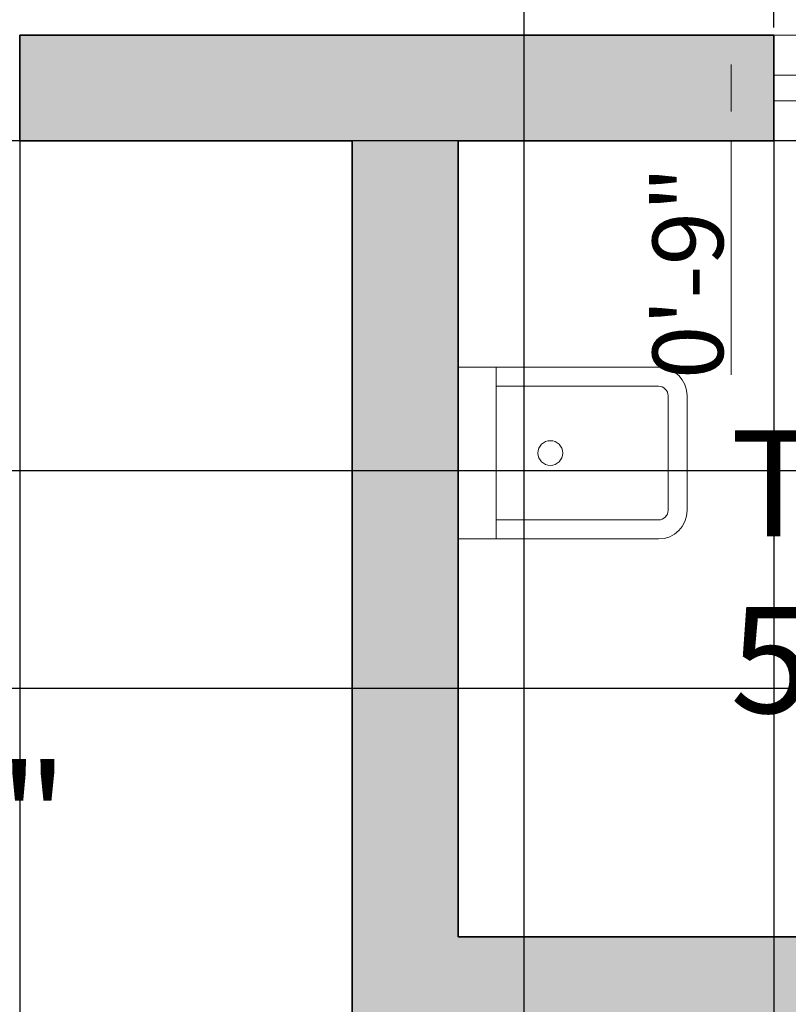
# Model space of a CAD drawing. Units: inches. Extents: x 2696 to 3240, y 1564 to 2310.
# Tile 54 of 76: x 2842 to 2907, y 2180 to 2264. Entities that reach past the tile are written whole.
import ezdxf

# ---------------------------------------------------------------- set-up
doc = ezdxf.new("R2010")
doc.units = ezdxf.units.IN
for name, color, linetype, lineweight in [('A-ANNO-DIMS', 3, 'Continuous', 18), ('A-AREA-IDEN', 7, 'Continuous', 18), ('A-FLOR-FIXT', 8, 'Continuous', 18), ('A-FURN', 251, 'Continuous', 13), ('A-WALL', 7, 'Continuous', 35), ('A-WALL-PATT', 9, 'Continuous', 13), ('WINDOW', 2, 'Continuous', 18)]:
    doc.layers.add(name, color=color, linetype=linetype, lineweight=lineweight)
doc.styles.add('TIMES NEW', font='times.ttf')
doc.styles.add('YQ_DIM', font='SUPEROS.SHX', dxfattribs={"width": 0.8, "bigfont": 'HZDX.SHX'})
doc.dimstyles.new('Siddhuu', dxfattribs={"dimtxt": 6, "dimasz": 2.5, "dimexe": 1.25, "dimexo": 0.625, "dimtad": 1, "dimdec": 1, "dimlunit": 4, "dimtxsty": 'TIMES NEW', "dimcen": 2.5, "dimclrd": 256, "dimclre": 1, "dimclrt": 7, "dimadec": 0, "dimazin": 0, "dimtfac": 1, "dimtdec": 1, "dimtmove": 0, "dimatfit": 3, "dimfxl": 1, "dimtolj": 1, "dimlwd": -1, "dimarcsym": 0})

# ---------------------------------------------------------------- blocks, each defined once
blk = doc.blocks.new('WD_WIN4')
for p, q in [((-0.5, 0.5), (0.5, 0.5)), ((-0.5, 0.12), (0.5, 0.12)), ((-0.5, -0.12), (0.5, -0.12)), ((-0.5, -0.5), (0.5, -0.5))]:
    blk.add_line(p, q)
blk = doc.blocks.new('*D9')
at = {"layer": 'A-ANNO-DIMS', "color": 0, "lineweight": -2, "transparency": 16777216}
for p, q in [((2745.611, 2262.826), (2745.611, 2282.188)), ((3199.611, 2262.826), (3199.611, 2282.188))]:
    blk.add_line(p, q, dxfattribs=at)
at = {"layer": 'A-ANNO-DIMS', "color": 0, "transparency": 16777216}
blk.add_line((2757.611, 2280.938), (3187.611, 2280.938), dxfattribs=at)
for points in [[(2757.611, 2282.938), (2757.611, 2278.938), (2745.611, 2280.938)], [(3187.611, 2282.938), (3187.611, 2278.938), (3199.611, 2280.938)]]:
    blk.add_solid(points, dxfattribs=at)
at = {"layer": 'Defpoints', "color": 0, "transparency": 16777216}
for p in [(3199.611, 2280.938), (2745.611, 2262.201), (3199.611, 2262.201)]:
    blk.add_point(p, dxfattribs=at)
at = {"layer": 'A-ANNO-DIMS', "color": 0, "transparency": 16777216, "insert": (2972.611, 2290.718), "char_height": 18, "attachment_point": 5, "style": 'TIMES NEW'}
blk.add_mtext("\\A1;36'", dxfattribs=at)
blk = doc.blocks.new('WC')
at = {"layer": 'A-FURN'}
for p, q in [((0, 14.59), (-17.022, 14.59)), ((-3.242, 14.59), (-3.242, 0)), ((-3.242, 12.969), (-17.022, 12.969)), ((-19.454, 2.432), (-19.454, 12.159)), ((-17.833, 2.432), (-17.833, 12.159)), ((-3.242, 1.621), (-17.022, 1.621)), ((0, 0), (-17.022, 0))]:
    blk.add_line(p, q, dxfattribs=at)
blk.add_circle((-7.836, 7.295), 1.051, dxfattribs=at)
for centre, radius, start, end in [((-17.022, 12.159), 2.432, 90, 180), ((-17.022, 12.159), 0.811, 90, 180), ((-17.022, 2.432), 2.432, 180, 270), ((-17.022, 2.432), 0.811, 180, 270)]:
    blk.add_arc(centre, radius, start, end, dxfattribs=at)
blk = doc.blocks.new('*D20')
at = {"layer": 'A-ANNO-DIMS', "color": 1, "lineweight": -2, "transparency": 16777216}
for p, q in [((2905.91, 2262.826), (2905.91, 2267.051)), ((2929.91, 2262.826), (2929.91, 2267.051))]:
    blk.add_line(p, q, dxfattribs=at)
at = {"layer": 'A-ANNO-DIMS', "transparency": 16777216}
for p, q in [((2905.91, 2265.801), (2844.76, 2265.801)), ((2927.41, 2265.801), (2908.41, 2265.801))]:
    blk.add_line(p, q, dxfattribs=at)
for points in [[(2908.41, 2266.218), (2908.41, 2265.384), (2905.91, 2265.801)], [(2927.41, 2266.218), (2927.41, 2265.384), (2929.91, 2265.801)]]:
    blk.add_solid(points, dxfattribs=at)
at = {"layer": 'Defpoints', "color": 0, "transparency": 16777216}
for p in [(2905.91, 2265.801), (2905.91, 2262.201), (2929.91, 2262.201)]:
    blk.add_point(p, dxfattribs=at)
at = {"layer": 'A-ANNO-DIMS', "color": 7, "transparency": 16777216, "insert": (2874.085, 2269.493), "char_height": 6, "attachment_point": 5, "style": 'TIMES NEW'}
blk.add_mtext('\\A1;WINDOW 2\'-0"', dxfattribs=at)
blk = doc.blocks.new('*D21')
at = {"layer": 'A-ANNO-DIMS', "color": 1, "lineweight": -2, "transparency": 16777216}
for p, q in [((2905.285, 2262.201), (2901.06, 2262.201)), ((2905.285, 2253.201), (2901.06, 2253.201))]:
    blk.add_line(p, q, dxfattribs=at)
at = {"layer": 'A-ANNO-DIMS', "transparency": 16777216}
for p, q in [((2902.31, 2259.701), (2902.31, 2255.701)), ((2902.31, 2253.201), (2902.31, 2233.337))]:
    blk.add_line(p, q, dxfattribs=at)
for points in [[(2901.893, 2259.701), (2902.727, 2259.701), (2902.31, 2262.201)], [(2901.893, 2255.701), (2902.727, 2255.701), (2902.31, 2253.201)]]:
    blk.add_solid(points, dxfattribs=at)
at = {"layer": 'Defpoints', "color": 0, "transparency": 16777216}
for p in [(2905.91, 2262.201), (2902.31, 2253.201), (2905.91, 2253.201)]:
    blk.add_point(p, dxfattribs=at)
at = {"layer": 'A-ANNO-DIMS', "color": 7, "transparency": 16777216, "insert": (2898.625, 2242.019), "char_height": 6, "attachment_point": 5, "rotation": 90, "style": 'TIMES NEW'}
blk.add_mtext('\\A1;0\'-9"', dxfattribs=at)
blk = doc.blocks.new('*D59')
at = {"layer": 'A-ANNO-DIMS', "color": 1, "lineweight": -2, "transparency": 16777216}
for p, q in [((2884.709, 1740.826), (2884.709, 2298.451)), ((2956.709, 1740.826), (2956.709, 2298.451))]:
    blk.add_line(p, q, dxfattribs=at)
at = {"layer": 'A-ANNO-DIMS', "transparency": 16777216}
blk.add_line((2887.209, 2297.201), (2954.209, 2297.201), dxfattribs=at)
for points in [[(2887.209, 2297.618), (2887.209, 2296.784), (2884.709, 2297.201)], [(2954.209, 2297.618), (2954.209, 2296.784), (2956.709, 2297.201)]]:
    blk.add_solid(points, dxfattribs=at)
at = {"layer": 'Defpoints', "color": 0, "transparency": 16777216}
for p in [(2956.709, 2297.201), (2884.709, 1740.201), (2956.709, 1740.201)]:
    blk.add_point(p, dxfattribs=at)
at = {"layer": 'A-ANNO-DIMS', "color": 7, "transparency": 16777216, "insert": (2920.709, 2300.878), "char_height": 6, "attachment_point": 5, "style": 'TIMES NEW'}
blk.add_mtext('\\A1;6\'-0"', dxfattribs=at)
blk = doc.blocks.new('*D64')
at = {"layer": 'A-ANNO-DIMS', "color": 1, "lineweight": -2, "transparency": 16777216}
for p, q in [((3073.084, 2206.701), (2709.361, 2206.701)), ((3068.584, 1989.201), (2709.361, 1989.201))]:
    blk.add_line(p, q, dxfattribs=at)
at = {"layer": 'A-ANNO-DIMS', "transparency": 16777216}
blk.add_line((2710.611, 1991.701), (2710.611, 2204.201), dxfattribs=at)
for points in [[(2710.195, 2204.201), (2711.028, 2204.201), (2710.611, 2206.701)], [(2710.195, 1991.701), (2711.028, 1991.701), (2710.611, 1989.201)]]:
    blk.add_solid(points, dxfattribs=at)
at = {"layer": 'Defpoints', "color": 0, "transparency": 16777216}
for p in [(2710.611, 2206.701), (3073.709, 2206.701), (3069.209, 1989.201)]:
    blk.add_point(p, dxfattribs=at)
at = {"layer": 'A-ANNO-DIMS', "color": 7, "transparency": 16777216, "insert": (2706.85, 2097.951), "char_height": 6, "attachment_point": 5, "rotation": 90, "style": 'TIMES NEW'}
blk.add_mtext('\\A1;18\'-1 1/2"', dxfattribs=at)
blk = doc.blocks.new('*D69')
at = {"layer": 'A-ANNO-DIMS', "color": 1, "lineweight": -2, "transparency": 16777216}
for p, q in [((2841.889, 2261.576), (2841.889, 1568.951)), ((2905.91, 2261.576), (2905.91, 1568.951))]:
    blk.add_line(p, q, dxfattribs=at)
at = {"layer": 'A-ANNO-DIMS', "transparency": 16777216}
blk.add_line((2844.389, 1570.201), (2903.41, 1570.201), dxfattribs=at)
for points in [[(2844.389, 1570.618), (2844.389, 1569.784), (2841.889, 1570.201)], [(2903.41, 1570.618), (2903.41, 1569.784), (2905.91, 1570.201)]]:
    blk.add_solid(points, dxfattribs=at)
at = {"layer": 'Defpoints', "color": 0, "transparency": 16777216}
for p in [(2841.889, 2262.201), (2905.91, 2262.201), (2905.91, 1570.201)]:
    blk.add_point(p, dxfattribs=at)
at = {"layer": 'A-ANNO-DIMS', "color": 7, "transparency": 16777216, "insert": (2873.9, 1573.878), "char_height": 6, "attachment_point": 5, "style": 'TIMES NEW'}
blk.add_mtext('\\A1;5\'-4"', dxfattribs=at)
blk = doc.blocks.new('*D76')
at = {"layer": 'A-ANNO-DIMS', "color": 1, "lineweight": -2, "transparency": 16777216}
for p, q in [((3189.986, 2253.201), (2709.361, 2253.201)), ((3189.986, 2225.201), (2709.361, 2225.201))]:
    blk.add_line(p, q, dxfattribs=at)
at = {"layer": 'A-ANNO-DIMS', "transparency": 16777216}
blk.add_line((2710.611, 2250.701), (2710.611, 2227.701), dxfattribs=at)
for points in [[(2710.195, 2250.701), (2711.028, 2250.701), (2710.611, 2253.201)], [(2710.195, 2227.701), (2711.028, 2227.701), (2710.611, 2225.201)]]:
    blk.add_solid(points, dxfattribs=at)
at = {"layer": 'Defpoints', "color": 0, "transparency": 16777216}
for p in [(3190.611, 2253.201), (2710.611, 2225.201), (3190.611, 2225.201)]:
    blk.add_point(p, dxfattribs=at)
at = {"layer": 'A-ANNO-DIMS', "color": 7, "transparency": 16777216, "insert": (2706.986, 2239.201), "char_height": 6, "attachment_point": 5, "rotation": 90, "style": 'TIMES NEW'}
blk.add_mtext('\\A1;2\'-4"', dxfattribs=at)

msp = doc.modelspace()

# ---------------------------------------------------------------- hatches: boundary and pattern name
at = {"layer": 'A-WALL-PATT', "transparency": 33554556}
h = msp.add_hatch(color=256, dxfattribs=at)
h.dxf.hatch_style = 1
h.paths.add_polyline_path([(2879.111, 2253.201), (2905.91, 2253.201), (2905.91, 2262.201), (2841.889, 2262.201), (2841.889, 2253.201), (2870.111, 2253.201), (2870.111, 2176.601), (2965.709, 2176.601), (2965.709, 2206.701), (2973.583, 2206.701), (2973.583, 2215.701), (2965.709, 2215.701), (2965.709, 2262.201), (2929.91, 2262.201), (2929.91, 2253.201), (2956.709, 2253.201), (2956.709, 2185.601), (2879.111, 2185.601)])
h.paths.add_polyline_path([(2782.834, 2262.201), (2745.611, 2262.201), (2745.611, 2228.729), (2754.611, 2228.729), (2754.611, 2253.201), (2782.834, 2253.201)])
h.paths.add_polyline_path([(2754.611, 2136.201), (2965.709, 2136.201), (2965.709, 2145.201), (2879.111, 2145.201), (2879.111, 2147.074), (2877.34, 2147.074), (2870.111, 2147.074), (2870.111, 2145.201), (2754.611, 2145.201), (2754.611, 2169.674), (2745.611, 2169.674), (2745.611, 2000.201), (2754.611, 2000.201), (2754.611, 2019.201), (2849.083, 2019.201), (2849.083, 2023.701), (2841.209, 2023.701), (2841.209, 2051.827), (2836.709, 2051.827), (2836.709, 2023.701), (2754.611, 2023.701), (2754.611, 2091.201), (2836.709, 2091.201), (2836.709, 2087.827), (2841.209, 2087.827), (2841.209, 2095.701), (2754.611, 2095.701)])
h.paths.add_polyline_path([(2965.709, 2136.201), (2956.709, 2136.201), (2956.709, 2023.701), (2885.083, 2023.701), (2885.083, 2019.201), (2956.709, 2019.201), (2956.709, 1950.575), (2965.709, 1950.575), (2965.709, 1980.201), (2973.583, 1980.201), (2973.583, 1989.201), (2965.709, 1989.201)])
h.paths.add_polyline_path([(2754.611, 1906.701), (2880.209, 1906.701), (2884.709, 1906.701), (2956.709, 1906.701), (2956.709, 1792.701), (2944.709, 1792.701), (2944.709, 1783.701), (2956.709, 1783.701), (2956.709, 1740.201), (2884.709, 1740.201), (2884.709, 1783.701), (2896.709, 1783.701), (2896.709, 1792.701), (2884.709, 1792.701), (2884.709, 1846.701), (2880.209, 1846.701), (2880.209, 1740.201), (2754.611, 1740.201), (2754.611, 1777.201), (2745.611, 1777.201), (2745.611, 1692.701), (2754.611, 1692.701), (2754.611, 1731.201), (2956.709, 1731.201), (2956.709, 1723.327), (2965.709, 1723.327), (2965.709, 1884.201), (2973.583, 1884.201), (2973.583, 1893.201), (2965.709, 1893.201), (2965.709, 1914.575), (2956.709, 1914.575), (2956.709, 1911.201), (2754.611, 1911.201), (2754.611, 1930.201), (2745.611, 1930.201), (2745.611, 1817.201), (2754.611, 1817.201), (2754.611, 1854.201), (2826.611, 1854.201), (2826.611, 1868.827), (2822.111, 1868.827), (2822.111, 1858.701), (2754.611, 1858.701)])
h.paths.add_polyline_path([(2965.709, 1656.201), (3008.237, 1656.201), (3008.237, 1665.201), (2965.709, 1665.201), (2965.709, 1693.327), (2956.709, 1693.327), (2956.709, 1686.201), (2934.583, 1686.201), (2934.583, 1681.701), (2956.709, 1681.701), (2956.709, 1614.201), (2896.709, 1614.201), (2896.709, 1681.701), (2904.583, 1681.701), (2904.583, 1686.201), (2892.209, 1686.201), (2892.209, 1614.201), (2858.41, 1614.201), (2858.41, 1605.201), (2965.709, 1605.201)])
h.paths.add_polyline_path([(2788.41, 1614.201), (2754.611, 1614.201), (2754.611, 1652.701), (2745.611, 1652.701), (2745.611, 1605.201), (2788.41, 1605.201)])
h.paths.add_polyline_path([(3199.611, 1633.048), (3190.611, 1633.048), (3190.611, 1614.201), (3082.611, 1614.201), (3082.611, 1665.201), (3070.237, 1665.201), (3070.237, 1656.201), (3078.111, 1656.201), (3078.111, 1605.201), (3199.611, 1605.201)])
h.paths.add_polyline_path([(3199.611, 1702.048), (3190.611, 1702.048), (3190.611, 1699.701), (3106.611, 1699.701), (3106.611, 1747.701), (3190.611, 1747.701), (3190.611, 1752.201), (3082.611, 1752.201), (3082.611, 1760.075), (3078.111, 1760.075), (3078.111, 1747.701), (3102.111, 1747.701), (3102.111, 1699.701), (3078.111, 1699.701), (3078.111, 1695.201), (3190.611, 1695.201), (3190.611, 1676.355), (3199.611, 1676.355)])
h.paths.add_polyline_path([(3199.611, 1783.201), (3190.611, 1783.201), (3190.611, 1745.355), (3199.611, 1745.355)])
h.paths.add_polyline_path([(3082.611, 1884.201), (3190.611, 1884.201), (3190.611, 1853.201), (3199.611, 1853.201), (3199.611, 1901.701), (3190.611, 1901.701), (3190.611, 1893.201), (3005.583, 1893.201), (3005.583, 1891.281), (3005.583, 1884.201), (3078.111, 1884.201), (3078.111, 1792.075), (3082.611, 1792.075)])
h.paths.add_polyline_path([(3199.611, 1994.701), (3190.611, 1994.701), (3190.611, 1989.201), (3073.709, 1989.201), (3073.709, 2034.201), (3069.209, 2034.201), (3069.209, 1989.201), (3005.583, 1989.201), (3005.583, 1980.201), (3190.611, 1980.201), (3190.611, 1971.701), (3199.611, 1971.701)])
h.paths.add_polyline_path([(3199.611, 2155.201), (3190.611, 2155.201), (3190.611, 2064.701), (3199.611, 2064.701)])
h.paths.add_polyline_path([(3190.611, 2074.701), (3106.611, 2074.701), (3106.611, 2122.701), (3190.611, 2122.701), (3190.611, 2127.201), (3082.709, 2127.201), (3082.709, 2135.075), (3073.709, 2135.075), (3073.709, 2122.701), (3102.111, 2122.701), (3102.111, 2074.701), (3069.209, 2074.701), (3069.209, 2070.201), (3190.611, 2070.201)])
h.paths.add_polyline_path([(3082.709, 2253.201), (3190.611, 2253.201), (3190.611, 2225.201), (3199.611, 2225.201), (3199.611, 2262.201), (3073.709, 2262.201), (3073.709, 2215.701), (3035.583, 2215.701), (3035.583, 2206.701), (3073.709, 2206.701), (3073.709, 2171.075), (3082.709, 2171.075)])

# ---------------------------------------------------------------- linework, layer by layer
at = {"layer": 'A-WALL'}
for p, q in [((2841.889, 2262.201), (2905.91, 2262.201)), ((2841.889, 2253.201), (2841.889, 2262.201)), ((2905.91, 2262.201), (2905.91, 2253.201)), ((2905.91, 2253.201), (2905.91, 2262.201)), ((2841.889, 2253.201), (2870.111, 2253.201)), ((2870.111, 2176.601), (2870.111, 2253.201)), ((2879.111, 2185.601), (2879.111, 2253.201)), ((2879.111, 2253.201), (2905.91, 2253.201)), ((2879.111, 2185.601), (2956.709, 2185.601))]:
    msp.add_line(p, q, dxfattribs=at)

# ---------------------------------------------------------------- block references
at = {"layer": 'A-FLOR-FIXT', "xscale": -1}
msp.add_blockref('WC', (2879.111, 2219.401), dxfattribs=at)
at = {"layer": 'WINDOW', "xscale": 24, "yscale": 9, "zscale": 24, "rotation": 180}
msp.add_blockref('WD_WIN4', (2917.91, 2257.701), dxfattribs=at)

# ---------------------------------------------------------------- texts
at = {"layer": 'A-AREA-IDEN', "char_height": 9, "attachment_point": 1, "style": 'YQ_DIM'}
for s, insert in [('TOILET\\P5\'X5\'4.5"', (2902.228, 2228.623)), ('BEDROOM\\P10\'4.5"X9\'0"', (2776.156, 2215.244))]:
    msp.add_mtext_dynamic_manual_height_columns(s, width=48.00324, gutter_width=12.5, heights=[0], dxfattribs=dict(at, insert=insert))

# ---------------------------------------------------------------- dimensions: what is measured, and where the dimension line sits
at = {"layer": 'A-ANNO-DIMS'}
for base, p1, p2, picture, middle in [((2956.709, 2297.201), (2884.709, 1740.201), (2956.709, 1740.201), '*D59', (2920.709, 2300.878)), ((2905.91, 1570.201), (2841.889, 2262.201), (2905.91, 2262.201), '*D69', (2873.9, 1573.878))]:
    dim = msp.add_linear_dim(base=base, p1=p1, p2=p2, dimstyle='Siddhuu', override={"dimdec": 1, "dimlfac": 1, "dimrnd": 0, "dimzin": 1, "dimdsep": 46, "dimlunit": 4, "dimfrac": 2}, dxfattribs=at)
    dim.commit()
    dim.dimension.update_dxf_attribs({"geometry": picture, "text_midpoint": middle})
dim = msp.add_linear_dim(base=(3199.611, 2280.938), p1=(2745.611, 2262.201), p2=(3199.611, 2262.201), text="36'", dimstyle='Siddhuu', override={"dimtxt": 18, "dimasz": 12, "dimclrd": 0, "dimclre": 0, "dimclrt": 0}, dxfattribs=at)
dim.commit()
dim.dimension.update_dxf_attribs({"geometry": '*D9', "text_midpoint": (2972.611, 2290.718)})
dim = msp.add_linear_dim(base=(2905.91, 2265.801), p1=(2929.91, 2262.201), p2=(2905.91, 2262.201), angle=180, text='WINDOW <>', dimstyle='Siddhuu', override={"dimdec": 1, "dimlfac": 1, "dimrnd": 0, "dimzin": 1, "dimdsep": 46, "dimlunit": 4, "dimfrac": 2}, dxfattribs=at)
dim.commit()
dim.dimension.update_dxf_attribs({"geometry": '*D20', "text_midpoint": (2874.085, 2269.493)})
for base, p1, p2, angle, picture, middle in [((2902.31, 2253.201), (2905.91, 2262.201), (2905.91, 2253.201), 270, '*D21', (2898.625, 2242.019)), ((2710.611, 2225.201), (3190.611, 2253.201), (3190.611, 2225.201), 90, '*D76', (2706.986, 2239.201)), ((2710.611, 2206.701), (3069.209, 1989.201), (3073.709, 2206.701), 90, '*D64', (2706.85, 2097.951))]:
    dim = msp.add_linear_dim(base=base, p1=p1, p2=p2, angle=angle, dimstyle='Siddhuu', override={"dimdec": 1, "dimlfac": 1, "dimrnd": 0, "dimzin": 1, "dimdsep": 46, "dimlunit": 4, "dimfrac": 2}, dxfattribs=at)
    dim.commit()
    dim.dimension.update_dxf_attribs({"geometry": picture, "text_midpoint": middle})

doc.saveas('drawing.dxf')
